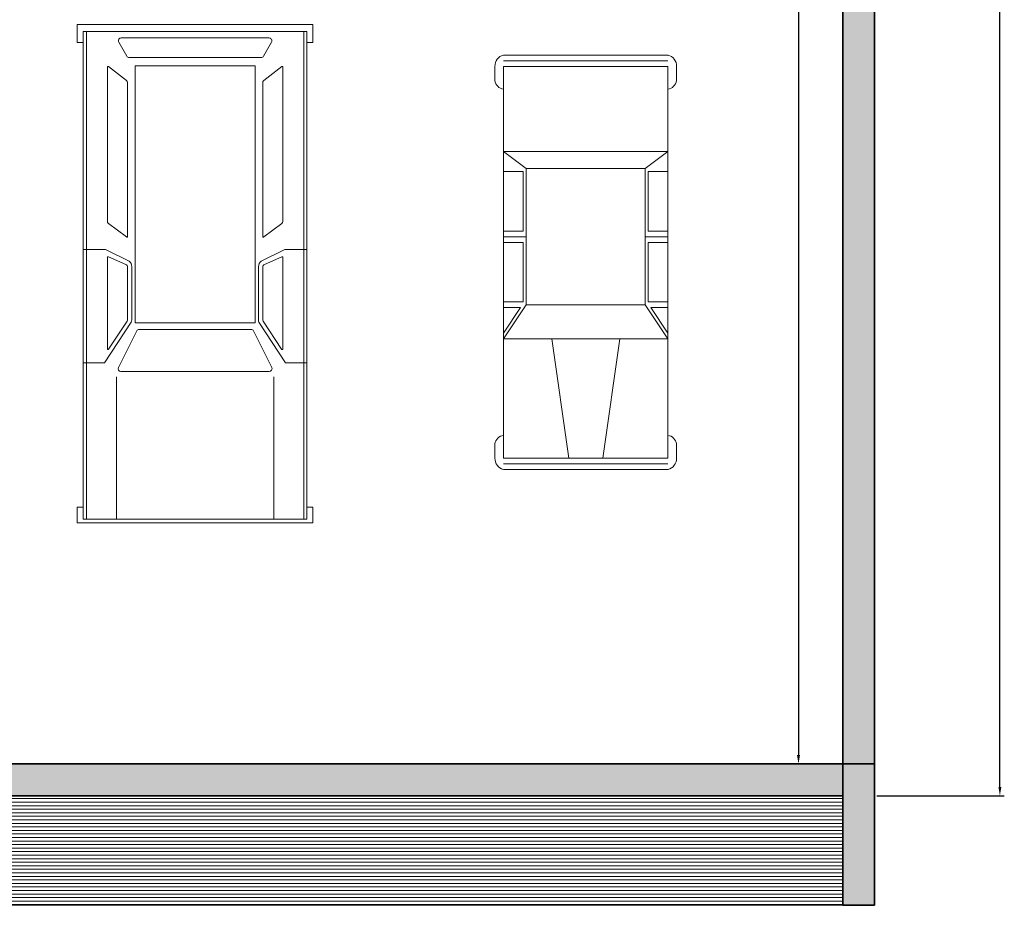
# Model space of a CAD drawing. Units: millimetres. Extents: x 2768 to 4359, y 795 to 1583.
# Tile 8 of 13: x 4080 to 4359, y 1008 to 1258. Entities that reach past the tile are written whole.
import ezdxf

# ---------------------------------------------------------------- set-up
doc = ezdxf.new("R2010")
doc.units = ezdxf.units.MM
for name, color, linetype, lineweight in [('A-ANNO-DIMS', 90, 'Continuous', 18), ('A-DOOR-PATT', 251, 'Continuous', 13), ('A-WALL-PATT', 140, 'Continuous', 9), ('C-PKNG-VEHI', 50, 'Continuous', 13), ('iron shutter', 251, 'Continuous', 18), ('walls', 140, 'Continuous', 35)]:
    doc.layers.add(name, color=color, linetype=linetype, lineweight=lineweight)
doc.styles.get("Standard").update_dxf_attribs({"font": 'arial.ttf'})
doc.dimstyles.new('ISO-25', dxfattribs={"dimtxt": 5, "dimasz": 2.5, "dimexe": 1.25, "dimexo": 0.625, "dimtad": 1, "dimdec": 0, "dimlunit": 3, "dimtxsty": 'Standard', "dimcen": 2.5, "dimadec": 0, "dimazin": 0, "dimtfac": 1, "dimtdec": 0, "dimtmove": 0, "dimatfit": 3, "dimfxl": 1, "dimarcsym": 0})

# ---------------------------------------------------------------- blocks, each defined once
blk = doc.blocks.new('*D67')
at = {"layer": 'A-ANNO-DIMS', "color": 0, "lineweight": -2, "transparency": 16777216}
for p, q in [((4301.96, 1531.81), (4299.57, 1531.81)), ((4300.82, 1529.31), (4300.82, 1050.31)), ((4301.96, 1047.81), (4299.57, 1047.81))]:
    blk.add_line(p, q, dxfattribs=at)
at = {"layer": 'A-ANNO-DIMS', "color": 0, "transparency": 16777216}
for points in [[(4300.4, 1529.31), (4301.24, 1529.31), (4300.82, 1531.81)], [(4300.4, 1050.31), (4301.24, 1050.31), (4300.82, 1047.81)]]:
    blk.add_solid(points, dxfattribs=at)
at = {"layer": 'Defpoints', "color": 0, "transparency": 16777216}
for p in [(4302.59, 1531.81), (4300.82, 1047.81), (4302.59, 1047.81)]:
    blk.add_point(p, dxfattribs=at)
at = {"layer": 'A-ANNO-DIMS', "color": 0, "transparency": 16777216, "insert": (4297.64, 1289.81), "char_height": 5, "attachment_point": 5, "rotation": 90}
blk.add_mtext('40\'-4"', dxfattribs=at)
blk = doc.blocks.new('*U35')
for p, q in [((5.44, 42.31), (12.12, 42.31)), ((189.69, 42.31), (183.01, 42.31)), ((0.1, -0.41), (0.1, 38.35)), ((2.77, -0.41), (2.77, 38.31)), ((5.44, -0.41), (5.44, 38.24)), ((5.45, 38.31), (16.12, 38.31)), ((16.12, 38.31), (180.34, 38.31)), ((61.52, -0.41), (61.52, 38.31)), ((61.52, 38.31), (77.54, 27.62)), ((64.19, 38.31), (76.2, 30.29)), ((76.2, 30.29), (76.2, 38.31)), ((78.87, 38.31), (78.87, 28.96)), ((106.91, 28.96), (106.91, 38.31)), ((109.58, 27.62), (109.58, 38.31)), ((112.25, 38.31), (112.25, 28.96)), ((140.29, 28.96), (140.29, 38.31)), ((141.62, 27.62), (149.64, 38.31)), ((149.64, -0.41), (149.64, 38.31)), ((189.69, 38.31), (179.01, 38.31)), ((189.69, -0.41), (189.69, 38.24)), ((192.36, -0.41), (192.36, 38.31)), ((195.03, -0.41), (195.03, 38.35)), ((78.87, 28.96), (106.91, 28.96)), ((112.25, 28.96), (140.29, 28.96)), ((77.54, 27.62), (141.62, 27.62)), ((77.54, -0.41), (77.54, 27.62)), ((141.62, -0.41), (141.62, 27.62)), ((5.44, 7.6), (61.52, 15.61)), ((0.1, -0.42), (0.1, -39.18)), ((2.77, -0.41), (2.77, -39.13)), ((5.44, -0.42), (5.44, -39.07)), ((61.52, -0.41), (61.52, -39.13)), ((77.54, -0.41), (77.54, -28.45)), ((141.62, -0.41), (141.62, -28.45)), ((149.64, -0.41), (149.64, -39.13)), ((189.69, -0.42), (189.69, -39.07)), ((192.36, -0.41), (192.36, -39.13)), ((195.03, -0.42), (195.03, -39.18)), ((5.44, -8.42), (61.52, -16.43)), ((61.52, -39.13), (77.54, -28.45)), ((64.19, -39.13), (76.2, -31.12)), ((76.2, -31.12), (76.2, -39.13)), ((77.54, -28.45), (141.62, -28.45)), ((78.87, -39.13), (78.87, -29.79)), ((78.87, -29.79), (106.91, -29.79)), ((106.91, -29.79), (106.91, -39.13)), ((109.58, -28.45), (109.58, -39.13)), ((112.25, -29.79), (140.29, -29.79)), ((112.25, -39.13), (112.25, -29.79)), ((140.29, -29.79), (140.29, -39.13)), ((141.62, -28.45), (149.64, -39.13)), ((5.45, -39.13), (16.12, -39.13)), ((16.12, -39.13), (180.34, -39.13)), ((189.69, -39.13), (179.01, -39.13)), ((5.44, -43.14), (12.12, -43.14)), ((189.69, -43.14), (183.01, -43.14))]:
    blk.add_line(p, q)
for centre, radius, start, end in [((5.06, 37.26), 5.06, 85.6455, 168.0943), ((11.45, 37.64), 4.72, 8.1301, 81.87), ((183.68, 37.64), 4.72, 98.13, 171.8699), ((190.07, 37.26), 5.06, 11.9057, 94.3545), ((5.06, -38.09), 5.06, 191.9057, 274.3545), ((11.45, -38.46), 4.72, 278.13, 351.8699), ((183.68, -38.46), 4.72, 188.1301, 261.87), ((190.07, -38.09), 5.06, 265.6455, 348.0943)]:
    blk.add_arc(centre, radius, start, end)
blk = doc.blocks.new('*U68')
for p, q in [((1.28, 38.87), (175.66, 38.87)), ((1.28, 28.15), (52.13, 28.15)), ((1.28, -28.15), (52.13, -28.15)), ((1.28, -38.87), (175.66, -38.87))]:
    blk.add_line(p, q)
for points in [[(5.57, 40.01), (5.57, 42.18), (0, 42.18), (0, -42.18), (5.57, -42.18), (5.57, -40.01), (1.28, -40.01), (1.28, 40.01)], [(1.28, 40.01), (175.66, 40.01), (175.66, -40.01), (1.28, -40.01)], [(171.74, 40.01), (175.66, 40.01), (175.66, -40.01), (171.74, -40.01), (171.74, -42.18), (178.14, -42.18), (178.14, 42.18), (171.74, 42.18)], [(71.47, 21.48), (163.42, 21.48), (163.42, -21.48), (71.47, -21.48)]]:
    blk.add_lwpolyline(points, close=True)
for points in [[(57.15, 40.01), (57.15, 32.39), (71.72, 22.83, 0.086577), (72.56, 22.68), (91.59, 22.68, 0.227875), (93.54, 23.62), (97.72, 32.11), (97.72, 40.01)], [(57.15, -40.01), (57.15, -32.39), (71.72, -22.83, -0.086577), (72.56, -22.68), (91.59, -22.68, -0.227875), (93.54, -23.62), (97.72, -32.11), (97.72, -40.01)]]:
    blk.add_lwpolyline(points, format="xyb")
for points in [[(62.08, 30.95), (72.14, 24.35, 0.146139), (72.69, 24.18), (91.42, 24.18, 0.29766), (92.33, 24.78), (95.09, 31.05, 0.541236), (94.86, 31.41), (62.21, 31.41, 0.744989)], [(102.19, 24.58), (106.97, 31, -0.236929), (107.78, 31.41), (162.91, 31.41, -0.621576), (163.11, 31), (158.19, 24.58, -0.233368), (157.39, 24.18), (102.39, 24.18, -0.616908)], [(55.49, 27.42), (68.59, 20.89, -0.284287), (69.14, 19.99), (69.14, -19.99, -0.284287), (68.59, -20.89), (55.49, -27.42, -0.557284), (54.05, -26.53), (54.05, 26.53, -0.557284)], [(171.88, 27.31), (166.83, 24.47, 0.271143), (166.32, 23.6), (166.32, -23.6, 0.271143), (166.83, -24.47), (171.88, -27.31, 0.573387), (173.37, -26.44), (173.37, 26.44, 0.573387)], [(62.08, -30.95), (72.14, -24.35, -0.146139), (72.69, -24.18), (91.42, -24.18, -0.29766), (92.33, -24.78), (95.09, -31.05, -0.541236), (94.86, -31.41), (62.21, -31.41, -0.744989)], [(102.19, -24.58), (106.97, -31, 0.236929), (107.78, -31.41), (162.91, -31.41, 0.621576), (163.11, -31), (158.19, -24.58, 0.233368), (157.39, -24.18), (102.39, -24.18, 0.616908)]]:
    blk.add_lwpolyline(points, format="xyb", close=True)
blk = doc.blocks.new('*D130')
at = {"layer": 'A-ANNO-DIMS', "color": 0, "lineweight": -2, "transparency": 16777216}
for p, q in [((4322.99, 1540.81), (4359.12, 1540.81)), ((4357.87, 1041.31), (4357.87, 1538.31)), ((4322.99, 1038.81), (4359.12, 1038.81))]:
    blk.add_line(p, q, dxfattribs=at)
at = {"layer": 'A-ANNO-DIMS', "color": 0, "transparency": 16777216}
for points in [[(4357.45, 1538.31), (4358.28, 1538.31), (4357.87, 1540.81)], [(4357.45, 1041.31), (4358.28, 1041.31), (4357.87, 1038.81)]]:
    blk.add_solid(points, dxfattribs=at)
at = {"layer": 'Defpoints', "color": 0, "transparency": 16777216}
for p in [(4322.37, 1540.81), (4357.87, 1540.81), (4322.37, 1038.81)]:
    blk.add_point(p, dxfattribs=at)
at = {"layer": 'A-ANNO-DIMS', "color": 0, "transparency": 16777216, "insert": (4354.69, 1289.81), "char_height": 5, "attachment_point": 5, "rotation": 90}
blk.add_mtext('41\'-10"', dxfattribs=at)

msp = doc.modelspace()

# ---------------------------------------------------------------- hatches: boundary and pattern name
at = {"layer": 'A-DOOR-PATT'}
h = msp.add_hatch(dxfattribs=at)
h.set_pattern_fill('ANSI31', color=256, scale=0.3149606, angle=-45, style=0)
h.paths.add_polyline_path([(4072.37, 1038.81), (4313.37, 1038.81), (4313.37, 1007.81), (4072.37, 1007.81)])
at = {"layer": 'A-WALL-PATT'}
h = msp.add_hatch(color=256, dxfattribs=at)
h.dxf.hatch_style = 1
h.paths.add_polyline_path([(4313.37, 1540.81), (4072.37, 1540.81), (4072.37, 1531.81), (4313.37, 1531.81)])
h.paths.add_polyline_path([(4072.37, 1540.81), (4063.37, 1540.81), (4063.37, 1531.81), (4072.37, 1531.81)])
h.paths.add_polyline_path([(4322.37, 1540.81), (4313.37, 1540.81), (4313.37, 1531.81), (4322.37, 1531.81)])
h.paths.add_polyline_path([(4322.37, 1531.81), (4313.37, 1531.81), (4313.37, 1378.81), (4313.37, 1047.81), (4322.37, 1047.81), (4322.37, 1378.81)])
h.paths.add_polyline_path([(4313.37, 1047.81), (4072.37, 1047.81), (4072.37, 1038.81), (4313.37, 1038.81)])
h = msp.add_hatch(color=256, dxfattribs=at)
h.dxf.hatch_style = 1
h.paths.add_polyline_path([(4313.37, 1007.81), (4322.37, 1007.81), (4322.37, 1047.81), (4313.37, 1047.81)])

# ---------------------------------------------------------------- linework, layer by layer
at = {"layer": 'iron shutter'}
for p, q in [((4072.37, 1038.81), (4313.37, 1038.81)), ((4322.37, 1038.81), (4322.37, 1038.81)), ((4072.37, 1007.81), (4313.37, 1007.81))]:
    msp.add_line(p, q, dxfattribs=at)
at = {"layer": 'walls'}
for p, q in [((4313.37, 1378.81), (4313.37, 1007.81)), ((4322.37, 1378.81), (4322.37, 1007.81)), ((3896.37, 1047.81), (4322.37, 1047.81)), ((3905.37, 1038.81), (4313.37, 1038.81)), ((4313.37, 1007.81), (4322.37, 1007.81))]:
    msp.add_line(p, q, dxfattribs=at)

# ---------------------------------------------------------------- block references
at = {"layer": 'C-PKNG-VEHI', "rotation": 90}
for name, p, xscale, yscale, zscale in [('*U68', (4129.92, 1116.09), 0.7914409048616003, 0.7914409048616003, 0.7914409048616003), ('*U35', (4240.3, 1131.13), 0.6015497955747826, 0.6015497955747826, 0.6015497955747826)]:
    msp.add_blockref(name, p, dxfattribs=dict(at, xscale=xscale, yscale=yscale, zscale=zscale))

# ---------------------------------------------------------------- dimensions: what is measured, and where the dimension line sits
at = {"layer": 'A-ANNO-DIMS'}
for base, p1, p2, override, picture, middle in [((4357.87, 1540.81), (4322.37, 1038.81), (4322.37, 1540.81), {"dimdec": 1, "dimlfac": 1, "dimrnd": 0, "dimzin": 1, "dimdsep": 46, "dimlunit": 4, "dimfrac": 2}, '*D130', (4354.69, 1289.81)), ((4300.82, 1047.81), (4302.59, 1531.81), (4302.59, 1047.81), {"dimclrd": 0, "dimclre": 0, "dimclrt": 0}, '*D67', (4297.64, 1289.81))]:
    dim = msp.add_linear_dim(base=base, p1=p1, p2=p2, angle=90, dimstyle='ISO-25', override=override, dxfattribs=at)
    dim.commit()
    dim.dimension.update_dxf_attribs({"geometry": picture, "text_midpoint": middle})

doc.saveas('drawing.dxf')
